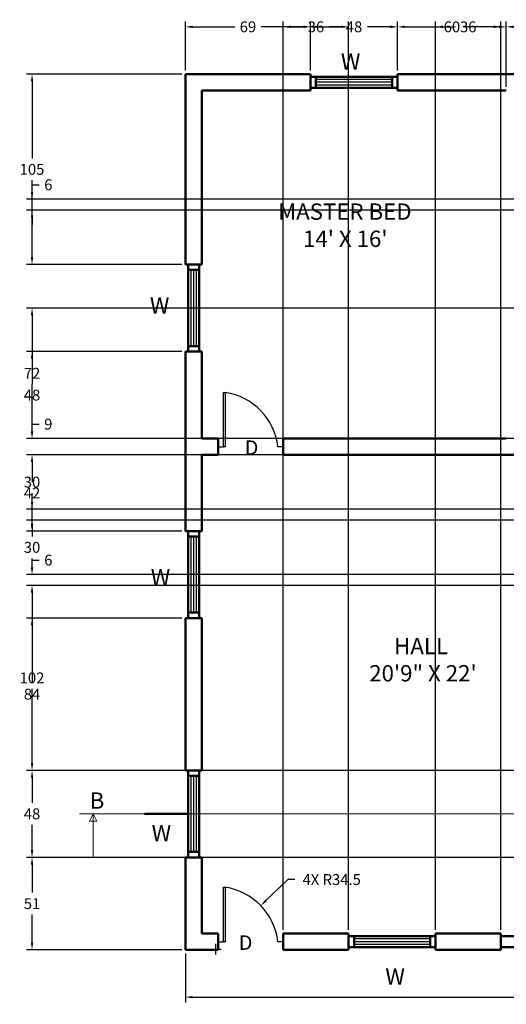
# Model space of a CAD drawing. Units: inches. Extents: x 853 to 2068, y 1026 to 2097.
# Tile 1 of 6: x 853 to 1122, y 1026 to 1569. Entities that reach past the tile are written whole.
import ezdxf

# ---------------------------------------------------------------- set-up
doc = ezdxf.new("R2010")
doc.units = ezdxf.units.IN
doc.header["$MEASUREMENT"] = 0
for name, color, linetype, lineweight in [('A-ANNO-DIMS', 2, 'Continuous', 18), ('A-ANNO-SYMB', 2, 'Continuous', 18), ('A-ANNO-TEXT', 3, 'Continuous', 18), ('A-AREA-IDEN', 7, 'Continuous', 18), ('A-DOOR', 3, 'Continuous', 25), ('A-GLAZ', 4, 'Continuous', 25), ('A-WALL', 7, 'Continuous', 50)]:
    doc.layers.add(name, color=color, linetype=linetype, lineweight=lineweight)
doc.styles.get("Standard").update_dxf_attribs({"font": 'arial.ttf'})
doc.dimstyles.get("Standard").update_dxf_attribs({"dimtxt": 6, "dimasz": 4, "dimexe": 3, "dimexo": 2, "dimgap": 3, "dimtad": 0, "dimtih": 1, "dimtoh": 1, "dimdec": 0, "dimzin": 0, "dimdsep": 46, "dimlunit": 3, "dimtxsty": 'Standard', "dimcen": 3, "dimadec": 0, "dimazin": 0, "dimtfac": 1, "dimtdec": 0, "dimtofl": 0, "dimtmove": 0, "dimatfit": 3, "dimfxl": 1, "dimtolj": 1, "dimtzin": 0, "dimarcsym": 0})

# ---------------------------------------------------------------- blocks, each defined once
blk = doc.blocks.new('DOOR-D')
for p, q in [((0, 36), (0, 33)), ((0, 33), (30, 33)), ((0, 32), (0, 33)), ((30, 33), (30, 32)), ((30, 32), (0, 32)), ((0, 0), (0, 3))]:
    blk.add_line(p, q)
blk.add_arc((-4.1, 37.26), 34.5, 276.8214, 351.2366)
blk = doc.blocks.new('*D13')
at = {"layer": 'A-ANNO-DIMS', "color": 0, "lineweight": -2, "transparency": 16777216}
for p, q in [((944.75, 1054.25), (944.75, 1027.15)), ((1340.75, 1054.25), (1340.75, 1027.15)), ((948.75, 1030.15), (1133.13, 1030.15)), ((1336.75, 1030.15), (1152.38, 1030.15))]:
    blk.add_line(p, q, dxfattribs=at)
at = {"layer": 'A-ANNO-DIMS', "color": 0, "transparency": 16777216}
for points in [[(948.75, 1030.82), (948.75, 1029.48), (944.75, 1030.15)], [(1336.75, 1030.82), (1336.75, 1029.48), (1340.75, 1030.15)]]:
    blk.add_solid(points, dxfattribs=at)
at = {"layer": 'Defpoints', "color": 0, "transparency": 16777216}
for p in [(944.75, 1056.25), (1340.75, 1056.25), (1340.75, 1030.15)]:
    blk.add_point(p, dxfattribs=at)
at = {"layer": 'A-ANNO-DIMS', "color": 0, "transparency": 16777216, "insert": (1142.75, 1030.15), "char_height": 6, "attachment_point": 5}
blk.add_mtext('\\A1;396', dxfattribs=at)
blk = doc.blocks.new('*D14')
at = {"layer": 'A-ANNO-DIMS', "color": 0, "lineweight": -2, "transparency": 16777216}
for p, q in [((998.75, 1067.25), (998.75, 1568.35)), ((1002.75, 1565.35), (1009.46, 1565.35)), ((1030.75, 1565.35), (1024.04, 1565.35)), ((1034.75, 1067.25), (1034.75, 1568.35))]:
    blk.add_line(p, q, dxfattribs=at)
at = {"layer": 'A-ANNO-DIMS', "color": 0, "transparency": 16777216}
for points in [[(1002.75, 1566.02), (1002.75, 1564.68), (998.75, 1565.35)], [(1030.75, 1566.02), (1030.75, 1564.68), (1034.75, 1565.35)]]:
    blk.add_solid(points, dxfattribs=at)
at = {"layer": 'Defpoints', "color": 0, "transparency": 16777216}
for p in [(1034.75, 1565.35), (998.75, 1065.25), (1034.75, 1065.25)]:
    blk.add_point(p, dxfattribs=at)
at = {"layer": 'A-ANNO-DIMS', "color": 0, "transparency": 16777216, "insert": (1016.75, 1565.35), "char_height": 6, "attachment_point": 5}
blk.add_mtext('\\A1;36', dxfattribs=at)
blk = doc.blocks.new('*D15')
at = {"layer": 'A-ANNO-DIMS', "color": 0, "lineweight": -2, "transparency": 16777216}
for p, q in [((1082.75, 1067.25), (1082.75, 1568.35)), ((1086.75, 1565.35), (1093.46, 1565.35)), ((1114.75, 1565.35), (1108.04, 1565.35)), ((1118.75, 1067.25), (1118.75, 1568.35))]:
    blk.add_line(p, q, dxfattribs=at)
at = {"layer": 'A-ANNO-DIMS', "color": 0, "transparency": 16777216}
for points in [[(1086.75, 1566.02), (1086.75, 1564.68), (1082.75, 1565.35)], [(1114.75, 1566.02), (1114.75, 1564.68), (1118.75, 1565.35)]]:
    blk.add_solid(points, dxfattribs=at)
at = {"layer": 'Defpoints', "color": 0, "transparency": 16777216}
for p in [(1118.75, 1565.35), (1082.75, 1065.25), (1118.75, 1065.25)]:
    blk.add_point(p, dxfattribs=at)
at = {"layer": 'A-ANNO-DIMS', "color": 0, "transparency": 16777216, "insert": (1100.75, 1565.35), "char_height": 6, "attachment_point": 5}
blk.add_mtext('\\A1;36', dxfattribs=at)
blk = doc.blocks.new('*D19')
at = {"layer": 'A-ANNO-DIMS', "color": 0, "lineweight": -2, "transparency": 16777216}
for p, q in [((944.75, 1541.25), (944.75, 1568.35)), ((948.75, 1565.35), (971.93, 1565.35)), ((1009.75, 1565.35), (986.57, 1565.35)), ((1013.75, 1541.25), (1013.75, 1568.35))]:
    blk.add_line(p, q, dxfattribs=at)
at = {"layer": 'A-ANNO-DIMS', "color": 0, "transparency": 16777216}
for points in [[(948.75, 1566.02), (948.75, 1564.68), (944.75, 1565.35)], [(1009.75, 1566.02), (1009.75, 1564.68), (1013.75, 1565.35)]]:
    blk.add_solid(points, dxfattribs=at)
at = {"layer": 'Defpoints', "color": 0, "transparency": 16777216}
for p in [(1013.75, 1565.35), (944.75, 1539.25), (1013.75, 1539.25)]:
    blk.add_point(p, dxfattribs=at)
at = {"layer": 'A-ANNO-DIMS', "color": 0, "transparency": 16777216, "insert": (979.25, 1565.35), "char_height": 6, "attachment_point": 5}
blk.add_mtext('\\A1;69', dxfattribs=at)
blk = doc.blocks.new('*D20')
at = {"layer": 'A-ANNO-DIMS', "color": 0, "lineweight": -2, "transparency": 16777216}
for p, q in [((1013.75, 1541.25), (1013.75, 1568.35)), ((1017.75, 1565.35), (1030.33, 1565.35)), ((1057.75, 1565.35), (1045.18, 1565.35)), ((1061.75, 1541.25), (1061.75, 1568.35))]:
    blk.add_line(p, q, dxfattribs=at)
at = {"layer": 'A-ANNO-DIMS', "color": 0, "transparency": 16777216}
for points in [[(1017.75, 1566.02), (1017.75, 1564.68), (1013.75, 1565.35)], [(1057.75, 1566.02), (1057.75, 1564.68), (1061.75, 1565.35)]]:
    blk.add_solid(points, dxfattribs=at)
at = {"layer": 'Defpoints', "color": 0, "transparency": 16777216}
for p in [(1061.75, 1565.35), (1013.75, 1539.25), (1061.75, 1539.25)]:
    blk.add_point(p, dxfattribs=at)
at = {"layer": 'A-ANNO-DIMS', "color": 0, "transparency": 16777216, "insert": (1037.75, 1565.35), "char_height": 6, "attachment_point": 5}
blk.add_mtext('\\A1;48', dxfattribs=at)
blk = doc.blocks.new('*D21')
at = {"layer": 'A-ANNO-DIMS', "color": 0, "lineweight": -2, "transparency": 16777216}
for p, q in [((1061.75, 1541.25), (1061.75, 1568.35)), ((1065.75, 1565.35), (1084.45, 1565.35)), ((1117.75, 1565.35), (1099.05, 1565.35)), ((1121.75, 1532.25), (1121.75, 1568.35))]:
    blk.add_line(p, q, dxfattribs=at)
at = {"layer": 'A-ANNO-DIMS', "color": 0, "transparency": 16777216}
for points in [[(1065.75, 1566.02), (1065.75, 1564.68), (1061.75, 1565.35)], [(1117.75, 1566.02), (1117.75, 1564.68), (1121.75, 1565.35)]]:
    blk.add_solid(points, dxfattribs=at)
at = {"layer": 'Defpoints', "color": 0, "transparency": 16777216}
for p in [(1121.75, 1565.35), (1061.75, 1539.25), (1121.75, 1530.25)]:
    blk.add_point(p, dxfattribs=at)
at = {"layer": 'A-ANNO-DIMS', "color": 0, "transparency": 16777216, "insert": (1091.75, 1565.35), "char_height": 6, "attachment_point": 5}
blk.add_mtext('\\A1;60', dxfattribs=at)
blk = doc.blocks.new('*D22')
at = {"layer": 'A-ANNO-DIMS', "color": 0, "lineweight": -2, "transparency": 16777216}
for p, q in [((1121.75, 1532.25), (1121.75, 1568.35)), ((1125.75, 1565.35), (1130.96, 1565.35)), ((1150.75, 1565.35), (1145.55, 1565.35)), ((1154.75, 1541.25), (1154.75, 1568.35))]:
    blk.add_line(p, q, dxfattribs=at)
at = {"layer": 'A-ANNO-DIMS', "color": 0, "transparency": 16777216}
for points in [[(1125.75, 1566.02), (1125.75, 1564.68), (1121.75, 1565.35)], [(1150.75, 1566.02), (1150.75, 1564.68), (1154.75, 1565.35)]]:
    blk.add_solid(points, dxfattribs=at)
at = {"layer": 'Defpoints', "color": 0, "transparency": 16777216}
for p in [(1154.75, 1565.35), (1154.75, 1539.25), (1121.75, 1530.25)]:
    blk.add_point(p, dxfattribs=at)
at = {"layer": 'A-ANNO-DIMS', "color": 0, "transparency": 16777216, "insert": (1138.25, 1565.35), "char_height": 6, "attachment_point": 5}
blk.add_mtext('\\A1;33', dxfattribs=at)
blk = doc.blocks.new('*D28')
at = {"layer": 'A-ANNO-DIMS', "color": 0, "lineweight": -2, "transparency": 16777216}
for p, q in [((942.75, 1107.25), (857.15, 1107.25)), ((860.15, 1103.25), (860.15, 1087.81)), ((860.15, 1060.25), (860.15, 1075.69)), ((942.75, 1056.25), (857.15, 1056.25))]:
    blk.add_line(p, q, dxfattribs=at)
at = {"layer": 'A-ANNO-DIMS', "color": 0, "transparency": 16777216}
for points in [[(859.48, 1103.25), (860.82, 1103.25), (860.15, 1107.25)], [(859.48, 1060.25), (860.82, 1060.25), (860.15, 1056.25)]]:
    blk.add_solid(points, dxfattribs=at)
at = {"layer": 'Defpoints', "color": 0, "transparency": 16777216}
for p in [(860.15, 1107.25), (944.75, 1107.25), (944.75, 1056.25)]:
    blk.add_point(p, dxfattribs=at)
at = {"layer": 'A-ANNO-DIMS', "color": 0, "transparency": 16777216, "insert": (860.15, 1081.75), "char_height": 6, "attachment_point": 5}
blk.add_mtext('\\A1;51', dxfattribs=at)
blk = doc.blocks.new('*D29')
at = {"layer": 'A-ANNO-DIMS', "color": 0, "lineweight": -2, "transparency": 16777216}
for p, q in [((942.75, 1239.25), (857.15, 1239.25)), ((860.15, 1235.25), (860.15, 1203.31)), ((860.15, 1159.25), (860.15, 1191.19)), ((942.75, 1155.25), (857.15, 1155.25))]:
    blk.add_line(p, q, dxfattribs=at)
at = {"layer": 'A-ANNO-DIMS', "color": 0, "transparency": 16777216}
for points in [[(859.48, 1235.25), (860.82, 1235.25), (860.15, 1239.25)], [(859.48, 1159.25), (860.82, 1159.25), (860.15, 1155.25)]]:
    blk.add_solid(points, dxfattribs=at)
at = {"layer": 'Defpoints', "color": 0, "transparency": 16777216}
for p in [(860.15, 1239.25), (944.75, 1239.25), (944.75, 1155.25)]:
    blk.add_point(p, dxfattribs=at)
at = {"layer": 'A-ANNO-DIMS', "color": 0, "transparency": 16777216, "insert": (860.15, 1197.25), "char_height": 6, "attachment_point": 5}
blk.add_mtext('\\A1;84', dxfattribs=at)
blk = doc.blocks.new('*D30')
at = {"layer": 'A-ANNO-DIMS', "color": 0, "lineweight": -2, "transparency": 16777216}
for p, q in [((951.75, 1329.25), (857.15, 1329.25)), ((860.15, 1325.25), (860.15, 1314.26)), ((860.15, 1291.25), (860.15, 1302.24)), ((942.75, 1287.25), (857.15, 1287.25))]:
    blk.add_line(p, q, dxfattribs=at)
at = {"layer": 'A-ANNO-DIMS', "color": 0, "transparency": 16777216}
for points in [[(859.48, 1325.25), (860.82, 1325.25), (860.15, 1329.25)], [(859.48, 1291.25), (860.82, 1291.25), (860.15, 1287.25)]]:
    blk.add_solid(points, dxfattribs=at)
at = {"layer": 'Defpoints', "color": 0, "transparency": 16777216}
for p in [(860.15, 1329.25), (953.75, 1329.25), (944.75, 1287.25)]:
    blk.add_point(p, dxfattribs=at)
at = {"layer": 'A-ANNO-DIMS', "color": 0, "transparency": 16777216, "insert": (860.15, 1308.25), "char_height": 6, "attachment_point": 5}
blk.add_mtext('\\A1;42', dxfattribs=at)
blk = doc.blocks.new('*D31')
at = {"layer": 'A-ANNO-DIMS', "color": 0, "lineweight": -2, "transparency": 16777216}
for p, q in [((860.15, 1342.25), (860.15, 1346.25)), ((860.15, 1346.25), (864.15, 1346.25)), ((951.75, 1338.25), (857.15, 1338.25)), ((951.75, 1329.25), (857.15, 1329.25)), ((860.15, 1325.25), (860.15, 1321.25))]:
    blk.add_line(p, q, dxfattribs=at)
at = {"layer": 'A-ANNO-DIMS', "color": 0, "transparency": 16777216}
for points in [[(859.48, 1342.25), (860.82, 1342.25), (860.15, 1338.25)], [(859.48, 1325.25), (860.82, 1325.25), (860.15, 1329.25)]]:
    blk.add_solid(points, dxfattribs=at)
at = {"layer": 'Defpoints', "color": 0, "transparency": 16777216}
for p in [(860.15, 1338.25), (953.75, 1338.25), (953.75, 1329.25)]:
    blk.add_point(p, dxfattribs=at)
at = {"layer": 'A-ANNO-DIMS', "color": 0, "transparency": 16777216, "insert": (869.12, 1346.25), "char_height": 6, "attachment_point": 5}
blk.add_mtext('\\A1;9', dxfattribs=at)
blk = doc.blocks.new('*D32')
at = {"layer": 'A-ANNO-DIMS', "color": 0, "lineweight": -2, "transparency": 16777216}
for p, q in [((942.75, 1386.25), (857.15, 1386.25)), ((860.15, 1382.25), (860.15, 1368.31)), ((860.15, 1342.25), (860.15, 1356.19)), ((951.75, 1338.25), (857.15, 1338.25))]:
    blk.add_line(p, q, dxfattribs=at)
at = {"layer": 'A-ANNO-DIMS', "color": 0, "transparency": 16777216}
for points in [[(859.48, 1382.25), (860.82, 1382.25), (860.15, 1386.25)], [(859.48, 1342.25), (860.82, 1342.25), (860.15, 1338.25)]]:
    blk.add_solid(points, dxfattribs=at)
at = {"layer": 'Defpoints', "color": 0, "transparency": 16777216}
for p in [(860.15, 1386.25), (944.75, 1386.25), (953.75, 1338.25)]:
    blk.add_point(p, dxfattribs=at)
at = {"layer": 'A-ANNO-DIMS', "color": 0, "transparency": 16777216, "insert": (860.15, 1362.25), "char_height": 6, "attachment_point": 5}
blk.add_mtext('\\A1;48', dxfattribs=at)
blk = doc.blocks.new('*D33')
at = {"layer": 'A-ANNO-DIMS', "color": 0, "lineweight": -2, "transparency": 16777216}
for p, q in [((942.75, 1539.25), (857.15, 1539.25)), ((860.15, 1535.25), (860.15, 1492.81)), ((860.15, 1438.25), (860.15, 1480.69)), ((942.75, 1434.25), (857.15, 1434.25))]:
    blk.add_line(p, q, dxfattribs=at)
at = {"layer": 'A-ANNO-DIMS', "color": 0, "transparency": 16777216}
for points in [[(859.48, 1535.25), (860.82, 1535.25), (860.15, 1539.25)], [(859.48, 1438.25), (860.82, 1438.25), (860.15, 1434.25)]]:
    blk.add_solid(points, dxfattribs=at)
at = {"layer": 'Defpoints', "color": 0, "transparency": 16777216}
for p in [(860.15, 1539.25), (944.75, 1539.25), (944.75, 1434.25)]:
    blk.add_point(p, dxfattribs=at)
at = {"layer": 'A-ANNO-DIMS', "color": 0, "transparency": 16777216, "insert": (860.15, 1486.75), "char_height": 6, "attachment_point": 5}
blk.add_mtext('\\A1;105', dxfattribs=at)
blk = doc.blocks.new('*D35')
at = {"layer": 'A-ANNO-DIMS', "color": 0, "lineweight": -2, "transparency": 16777216}
for p, q in [((1329.75, 1155.25), (857.15, 1155.25)), ((860.15, 1151.25), (860.15, 1137.31)), ((860.15, 1111.25), (860.15, 1125.19)), ((1329.75, 1107.25), (857.15, 1107.25))]:
    blk.add_line(p, q, dxfattribs=at)
at = {"layer": 'A-ANNO-DIMS', "color": 0, "transparency": 16777216}
for points in [[(859.48, 1151.25), (860.82, 1151.25), (860.15, 1155.25)], [(859.48, 1111.25), (860.82, 1111.25), (860.15, 1107.25)]]:
    blk.add_solid(points, dxfattribs=at)
at = {"layer": 'Defpoints', "color": 0, "transparency": 16777216}
for p in [(860.15, 1155.25), (1331.75, 1155.25), (1331.75, 1107.25)]:
    blk.add_point(p, dxfattribs=at)
at = {"layer": 'A-ANNO-DIMS', "color": 0, "transparency": 16777216, "insert": (860.15, 1131.25), "char_height": 6, "attachment_point": 5}
blk.add_mtext('\\A1;48', dxfattribs=at)
blk = doc.blocks.new('*D36')
at = {"layer": 'A-ANNO-DIMS', "color": 0, "lineweight": -2, "transparency": 16777216}
for p, q in [((1329.75, 1257.25), (857.15, 1257.25)), ((860.15, 1253.25), (860.15, 1212.31)), ((860.15, 1159.25), (860.15, 1200.19)), ((1329.75, 1155.25), (857.15, 1155.25))]:
    blk.add_line(p, q, dxfattribs=at)
at = {"layer": 'A-ANNO-DIMS', "color": 0, "transparency": 16777216}
for points in [[(859.48, 1253.25), (860.82, 1253.25), (860.15, 1257.25)], [(859.48, 1159.25), (860.82, 1159.25), (860.15, 1155.25)]]:
    blk.add_solid(points, dxfattribs=at)
at = {"layer": 'Defpoints', "color": 0, "transparency": 16777216}
for p in [(860.15, 1257.25), (1331.75, 1257.25), (1331.75, 1155.25)]:
    blk.add_point(p, dxfattribs=at)
at = {"layer": 'A-ANNO-DIMS', "color": 0, "transparency": 16777216, "insert": (860.15, 1206.25), "char_height": 6, "attachment_point": 5}
blk.add_mtext('\\A1;102', dxfattribs=at)
blk = doc.blocks.new('*D37')
at = {"layer": 'A-ANNO-DIMS', "color": 0, "lineweight": -2, "transparency": 16777216}
for p, q in [((860.15, 1267.25), (860.15, 1271.25)), ((860.15, 1271.25), (864.15, 1271.25)), ((1329.75, 1263.25), (857.15, 1263.25)), ((1329.75, 1257.25), (857.15, 1257.25)), ((860.15, 1253.25), (860.15, 1249.25))]:
    blk.add_line(p, q, dxfattribs=at)
at = {"layer": 'A-ANNO-DIMS', "color": 0, "transparency": 16777216}
for points in [[(859.48, 1267.25), (860.82, 1267.25), (860.15, 1263.25)], [(859.48, 1253.25), (860.82, 1253.25), (860.15, 1257.25)]]:
    blk.add_solid(points, dxfattribs=at)
at = {"layer": 'Defpoints', "color": 0, "transparency": 16777216}
for p in [(860.15, 1263.25), (1331.75, 1263.25), (1331.75, 1257.25)]:
    blk.add_point(p, dxfattribs=at)
at = {"layer": 'A-ANNO-DIMS', "color": 0, "transparency": 16777216, "insert": (869.13, 1271.25), "char_height": 6, "attachment_point": 5}
blk.add_mtext('\\A1;6', dxfattribs=at)
blk = doc.blocks.new('*D38')
at = {"layer": 'A-ANNO-DIMS', "color": 0, "lineweight": -2, "transparency": 16777216}
for p, q in [((1329.75, 1410.25), (857.15, 1410.25)), ((860.15, 1406.25), (860.15, 1380.26)), ((860.15, 1342.25), (860.15, 1368.24)), ((1329.75, 1338.25), (857.15, 1338.25))]:
    blk.add_line(p, q, dxfattribs=at)
at = {"layer": 'A-ANNO-DIMS', "color": 0, "transparency": 16777216}
for points in [[(859.48, 1406.25), (860.82, 1406.25), (860.15, 1410.25)], [(859.48, 1342.25), (860.82, 1342.25), (860.15, 1338.25)]]:
    blk.add_solid(points, dxfattribs=at)
at = {"layer": 'Defpoints', "color": 0, "transparency": 16777216}
for p in [(860.15, 1410.25), (1331.75, 1410.25), (1331.75, 1338.25)]:
    blk.add_point(p, dxfattribs=at)
at = {"layer": 'A-ANNO-DIMS', "color": 0, "transparency": 16777216, "insert": (860.15, 1374.25), "char_height": 6, "attachment_point": 5}
blk.add_mtext('\\A1;72', dxfattribs=at)
blk = doc.blocks.new('*D39')
at = {"layer": 'A-ANNO-DIMS', "color": 0, "lineweight": -2, "transparency": 16777216}
for p, q in [((860.15, 1474.25), (860.15, 1478.25)), ((860.15, 1478.25), (864.15, 1478.25)), ((1200.75, 1470.25), (857.15, 1470.25)), ((1200.75, 1464.25), (857.15, 1464.25)), ((860.15, 1460.25), (860.15, 1456.25))]:
    blk.add_line(p, q, dxfattribs=at)
at = {"layer": 'A-ANNO-DIMS', "color": 0, "transparency": 16777216}
for points in [[(859.48, 1474.25), (860.82, 1474.25), (860.15, 1470.25)], [(859.48, 1460.25), (860.82, 1460.25), (860.15, 1464.25)]]:
    blk.add_solid(points, dxfattribs=at)
at = {"layer": 'Defpoints', "color": 0, "transparency": 16777216}
for p in [(860.15, 1470.25), (1202.75, 1470.25), (1202.75, 1464.25)]:
    blk.add_point(p, dxfattribs=at)
at = {"layer": 'A-ANNO-DIMS', "color": 0, "transparency": 16777216, "insert": (869.13, 1478.25), "char_height": 6, "attachment_point": 5}
blk.add_mtext('\\A1;6', dxfattribs=at)
blk = doc.blocks.new('*D43')
at = {"layer": 'A-ANNO-DIMS', "color": 0, "lineweight": -2, "transparency": 16777216}
for p, q in [((1230.75, 1293.25), (857.15, 1293.25)), ((860.15, 1289.25), (860.15, 1284.32)), ((860.15, 1267.25), (860.15, 1272.19)), ((1230.75, 1263.25), (857.15, 1263.25))]:
    blk.add_line(p, q, dxfattribs=at)
at = {"layer": 'A-ANNO-DIMS', "color": 0, "transparency": 16777216}
for points in [[(859.48, 1289.25), (860.82, 1289.25), (860.15, 1293.25)], [(859.48, 1267.25), (860.82, 1267.25), (860.15, 1263.25)]]:
    blk.add_solid(points, dxfattribs=at)
at = {"layer": 'Defpoints', "color": 0, "transparency": 16777216}
for p in [(860.15, 1293.25), (1232.75, 1293.25), (1232.75, 1263.25)]:
    blk.add_point(p, dxfattribs=at)
at = {"layer": 'A-ANNO-DIMS', "color": 0, "transparency": 16777216, "insert": (860.15, 1278.25), "char_height": 6, "attachment_point": 5}
blk.add_mtext('\\A1;30', dxfattribs=at)
blk = doc.blocks.new('*D44')
at = {"layer": 'A-ANNO-DIMS', "color": 0, "lineweight": -2, "transparency": 16777216}
for p, q in [((1230.75, 1329.25), (857.15, 1329.25)), ((860.15, 1325.25), (860.15, 1320.32)), ((860.15, 1303.25), (860.15, 1308.19)), ((1230.75, 1299.25), (857.15, 1299.25))]:
    blk.add_line(p, q, dxfattribs=at)
at = {"layer": 'A-ANNO-DIMS', "color": 0, "transparency": 16777216}
for points in [[(859.48, 1325.25), (860.82, 1325.25), (860.15, 1329.25)], [(859.48, 1303.25), (860.82, 1303.25), (860.15, 1299.25)]]:
    blk.add_solid(points, dxfattribs=at)
at = {"layer": 'Defpoints', "color": 0, "transparency": 16777216}
for p in [(860.15, 1329.25), (1232.75, 1329.25), (1232.75, 1299.25)]:
    blk.add_point(p, dxfattribs=at)
at = {"layer": 'A-ANNO-DIMS', "color": 0, "transparency": 16777216, "insert": (860.15, 1314.25), "char_height": 6, "attachment_point": 5}
blk.add_mtext('\\A1;30', dxfattribs=at)
blk = doc.blocks.new('*D115')
at = {"layer": 'A-ANNO-DIMS', "color": 0, "lineweight": -2, "transparency": 16777216}
for p, q in [((1001.18, 1095.02), (989.18, 1083.41)), ((1005.18, 1095.02), (1001.18, 1095.02)), ((961.49, 1053.65), (961.49, 1059.65)), ((958.49, 1056.65), (964.49, 1056.65))]:
    blk.add_line(p, q, dxfattribs=at)
at = {"layer": 'A-ANNO-DIMS', "color": 0, "transparency": 16777216}
blk.add_solid([(988.71, 1083.89), (989.64, 1082.93), (986.3, 1080.63)], dxfattribs=at)
at = {"layer": 'Defpoints', "color": 0, "transparency": 16777216}
for p in [(986.3, 1080.63), (961.49, 1056.65)]:
    blk.add_point(p, dxfattribs=at)
at = {"layer": 'A-ANNO-DIMS', "color": 0, "transparency": 16777216, "insert": (1025.44, 1095.02), "char_height": 6, "attachment_point": 5}
blk.add_mtext('\\A1;4X R34.5', dxfattribs=at)

msp = doc.modelspace()

# ---------------------------------------------------------------- linework, layer by layer
at = {"layer": 'A-ANNO-SYMB'}
for p, q in [((886.251, 1131.2513), (1399.251, 1131.2513)), ((891.8401, 1127.2513), (893.8401, 1131.2513)), ((893.8401, 1131.2513), (893.8401, 1107.2513)), ((893.8401, 1131.2513), (893.8401, 1127.2513)), ((895.8401, 1127.2513), (893.8401, 1131.2513)), ((893.8401, 1131.2513), (893.8401, 1127.2513)), ((893.8401, 1127.2513), (891.8401, 1127.2513)), ((893.8401, 1127.2513), (895.8401, 1127.2513))]:
    msp.add_line(p, q, dxfattribs=at)
at = {"layer": 'A-GLAZ'}
for p, q in [((1058.751, 1536.2513), (1016.751, 1536.2513)), ((1058.751, 1534.7513), (1016.751, 1534.7513)), ((1058.751, 1533.2513), (1016.751, 1533.2513)), ((947.751, 1431.2513), (947.751, 1389.2513)), ((949.251, 1431.2513), (949.251, 1389.2513)), ((950.751, 1431.2513), (950.751, 1389.2513)), ((947.751, 1284.2513), (947.751, 1242.2513)), ((949.251, 1284.2513), (949.251, 1242.2513)), ((950.751, 1284.2513), (950.751, 1242.2513)), ((947.751, 1152.2513), (947.751, 1110.2513)), ((949.251, 1152.2513), (949.251, 1110.2513)), ((950.751, 1152.2513), (950.751, 1110.2513)), ((1079.751, 1062.2513), (1037.751, 1062.2513)), ((1079.751, 1060.7513), (1037.751, 1060.7513)), ((1079.751, 1059.2513), (1037.751, 1059.2513))]:
    msp.add_line(p, q, dxfattribs=at)
at = {"layer": 'A-WALL'}
for p, q in [((944.751, 1539.2513), (1013.751, 1539.2513)), ((944.751, 1434.2513), (944.751, 1539.2513)), ((1013.751, 1539.2513), (1013.751, 1530.2513)), ((1061.751, 1537.7513), (1013.751, 1537.7513)), ((1016.751, 1537.7513), (1016.751, 1531.7513)), ((1058.751, 1537.7513), (1058.751, 1531.7513)), ((1061.751, 1539.2513), (1061.751, 1530.2513)), ((1061.751, 1539.2513), (1154.751, 1539.2513)), ((1061.751, 1531.7513), (1013.751, 1531.7513)), ((953.751, 1530.2513), (1013.751, 1530.2513)), ((953.751, 1530.2513), (1013.751, 1530.2513)), ((953.751, 1434.2513), (953.751, 1530.2513)), ((953.751, 1434.2513), (953.751, 1530.2513)), ((1061.751, 1530.2513), (1121.751, 1530.2513)), ((1061.751, 1530.2513), (1121.751, 1530.2513)), ((944.751, 1434.2513), (953.751, 1434.2513)), ((946.251, 1434.2513), (946.251, 1386.2513)), ((952.251, 1434.2513), (952.251, 1386.2513)), ((946.251, 1431.2513), (952.251, 1431.2513)), ((944.751, 1386.2513), (953.751, 1386.2513)), ((944.751, 1287.2513), (944.751, 1386.2513)), ((946.251, 1389.2513), (952.251, 1389.2513)), ((953.751, 1338.2513), (953.751, 1386.2513)), ((962.751, 1338.2513), (953.751, 1338.2513)), ((962.751, 1338.2513), (962.751, 1329.2513)), ((1121.751, 1338.2513), (998.751, 1338.2513)), ((998.751, 1338.2513), (998.751, 1329.2513)), ((953.751, 1329.2513), (953.751, 1287.2513)), ((962.751, 1329.2513), (953.751, 1329.2513)), ((953.751, 1287.2513), (953.751, 1329.2513)), ((1133.751, 1329.2513), (998.751, 1329.2513)), ((944.751, 1287.2513), (953.751, 1287.2513)), ((946.251, 1287.2513), (946.251, 1239.2513)), ((952.251, 1287.2513), (952.251, 1239.2513)), ((946.251, 1284.2513), (952.251, 1284.2513)), ((944.751, 1239.2513), (953.751, 1239.2513)), ((944.751, 1155.2513), (944.751, 1239.2513)), ((946.251, 1242.2513), (952.251, 1242.2513)), ((953.751, 1155.2513), (953.751, 1239.2513)), ((953.751, 1239.2513), (953.751, 1155.2513)), ((944.751, 1155.2513), (953.751, 1155.2513)), ((946.251, 1155.2513), (946.251, 1107.2513)), ((946.251, 1152.2513), (952.251, 1152.2513)), ((952.251, 1155.2513), (952.251, 1107.2513)), ((946.251, 1131.2513), (922.251, 1131.2513)), ((946.251, 1110.2513), (952.251, 1110.2513)), ((944.751, 1056.2513), (944.751, 1107.2513)), ((944.751, 1107.2513), (953.751, 1107.2513)), ((953.751, 1065.2513), (953.751, 1107.2513)), ((953.751, 1107.2513), (953.751, 1065.2513)), ((953.751, 1065.2513), (962.751, 1065.2513)), ((962.751, 1065.2513), (962.751, 1056.2513)), ((998.751, 1065.2513), (998.751, 1056.2513)), ((998.751, 1065.2513), (1034.751, 1065.2513)), ((1034.751, 1065.2513), (1034.751, 1056.2513)), ((1082.751, 1065.2513), (1082.751, 1056.2513)), ((1082.751, 1065.2513), (1082.751, 1056.2513)), ((1082.751, 1065.2513), (1118.751, 1065.2513)), ((1118.751, 1065.2513), (1118.751, 1056.2513)), ((1118.751, 1065.2513), (1118.751, 1056.2513)), ((1082.751, 1063.7513), (1034.751, 1063.7513)), ((1037.751, 1063.7513), (1037.751, 1057.7513)), ((1079.751, 1063.7513), (1079.751, 1057.7513)), ((1166.751, 1063.7513), (1118.751, 1063.7513)), ((944.751, 1056.2513), (962.751, 1056.2513)), ((998.751, 1056.2513), (1034.751, 1056.2513)), ((1082.751, 1057.7513), (1034.751, 1057.7513)), ((1082.751, 1056.2513), (1118.751, 1056.2513)), ((1166.751, 1057.7513), (1118.751, 1057.7513))]:
    msp.add_line(p, q, dxfattribs=at)

# ---------------------------------------------------------------- block references
at = {"layer": 'A-DOOR'}
for p, rotation in [((998.7513, 1333.7513), 90), ((998.7513, 1060.7513), 90.00000000000043)]:
    msp.add_blockref('DOOR-D', p, dxfattribs=dict(at, rotation=rotation))

# ---------------------------------------------------------------- texts
at = {"layer": 'A-ANNO-TEXT', "attachment_point": 1}
for s, insert, char_height in [('W', (1030.4812, 1550.7548), 9), ('W', (925.1273, 1416.2013), 9), ('D', (977.4841, 1337.2642), 8), ('W', (925.611, 1266.2835), 9), ('{\\fArial|b1|i0|c0|p34;B}', (891.9384, 1143.0903), 9), ('W', (926.0944, 1125.1936), 9), ('D', (974.2031, 1064.2336), 8), ('W', (1055.0353, 1046.0098), 9)]:
    msp.add_mtext_dynamic_manual_height_columns(s, width=85.037544, gutter_width=1, heights=[0], dxfattribs=dict(at, insert=insert, char_height=char_height))
at = {"layer": 'A-AREA-IDEN', "char_height": 9, "attachment_point": 1}
for s, insert in [("MASTER BED\\P     14' X 16'", (995.8748, 1467.9284)), ('     HALL\\P20\'9" X 22\'', (1046.1427, 1228.2964))]:
    msp.add_mtext_dynamic_manual_height_columns(s, width=85.037544, gutter_width=1, heights=[0], dxfattribs=dict(at, insert=insert))

# ---------------------------------------------------------------- dimensions: what is measured, and where the dimension line sits
at = {"layer": 'A-ANNO-DIMS'}
for base, p1, p2, picture, middle in [((1013.751, 1565.3513), (944.751, 1539.2513), (1013.751, 1539.2513), '*D19', (979.251, 1565.3513)), ((1034.751, 1565.3513), (998.751, 1065.2513), (1034.751, 1065.2513), '*D14', (1016.751, 1565.3513)), ((1061.751, 1565.3513), (1013.751, 1539.2513), (1061.751, 1539.2513), '*D20', (1037.751, 1565.3513)), ((1121.751, 1565.3513), (1061.751, 1539.2513), (1121.751, 1530.2513), '*D21', (1091.751, 1565.3513)), ((1118.751, 1565.3513), (1082.751, 1065.2513), (1118.751, 1065.2513), '*D15', (1100.751, 1565.3513)), ((1154.751, 1565.3513), (1121.751, 1530.2513), (1154.751, 1539.2513), '*D22', (1138.251, 1565.3513)), ((1340.751, 1030.1513), (944.751, 1056.2513), (1340.751, 1056.2513), '*D13', (1142.751, 1030.1513))]:
    dim = msp.add_linear_dim(base=base, p1=p1, p2=p2, dimstyle='Standard', override={"dimdec": 0, "dimlfac": 1, "dimrnd": 0, "dimzin": 0, "dimdsep": 46, "dimlunit": 2}, dxfattribs=at)
    dim.commit()
    dim.dimension.update_dxf_attribs({"geometry": picture, "text_midpoint": middle})
for base, p1, p2, picture, middle in [((860.151, 1539.2513), (944.751, 1434.2513), (944.751, 1539.2513), '*D33', (860.151, 1486.7513)), ((860.151, 1470.2513), (1202.751, 1464.2513), (1202.751, 1470.2513), '*D39', (869.1319, 1478.2513)), ((860.151, 1410.2513), (1331.751, 1338.2513), (1331.751, 1410.2513), '*D38', (860.151, 1374.2513)), ((860.151, 1386.2513), (953.751, 1338.2513), (944.751, 1386.2513), '*D32', (860.151, 1362.2513)), ((860.151, 1338.2513), (953.751, 1329.2513), (953.751, 1338.2513), '*D31', (869.1237, 1346.2513)), ((860.151, 1329.2513), (944.751, 1287.2513), (953.751, 1329.2513), '*D30', (860.151, 1308.2513)), ((860.151, 1329.2513), (1232.751, 1299.2513), (1232.751, 1329.2513), '*D44', (860.151, 1314.2513)), ((860.151, 1293.2513), (1232.751, 1263.2513), (1232.751, 1293.2513), '*D43', (860.151, 1278.2513)), ((860.151, 1263.2513), (1331.751, 1257.2513), (1331.751, 1263.2513), '*D37', (869.1319, 1271.2513)), ((860.151, 1257.2513), (1331.751, 1155.2513), (1331.751, 1257.2513), '*D36', (860.151, 1206.2513)), ((860.151, 1239.2513), (944.751, 1155.2513), (944.751, 1239.2513), '*D29', (860.151, 1197.2513)), ((860.151, 1155.2513), (1331.751, 1107.2513), (1331.751, 1155.2513), '*D35', (860.151, 1131.2513)), ((860.151, 1107.2513), (944.751, 1056.2513), (944.751, 1107.2513), '*D28', (860.151, 1081.7513))]:
    dim = msp.add_linear_dim(base=base, p1=p1, p2=p2, angle=90, dimstyle='Standard', override={"dimdec": 0, "dimlfac": 1, "dimrnd": 0, "dimzin": 0, "dimdsep": 46, "dimlunit": 2}, dxfattribs=at)
    dim.commit()
    dim.dimension.update_dxf_attribs({"geometry": picture, "text_midpoint": middle})
dim = msp.add_radius_dim(center=(961.4947, 1056.6535), mpoint=(986.3002, 1080.6322), text='4X <>', dimstyle='Standard', override={"dimdec": 1, "dimlfac": 1, "dimrnd": 0, "dimzin": 0, "dimdsep": 46, "dimlunit": 2}, dxfattribs=at)
dim.commit()
dim.dimension.update_dxf_attribs({"geometry": '*D115', "text_midpoint": (1025.4365, 1095.0193), "dimtype": 164})

doc.saveas('drawing.dxf')
